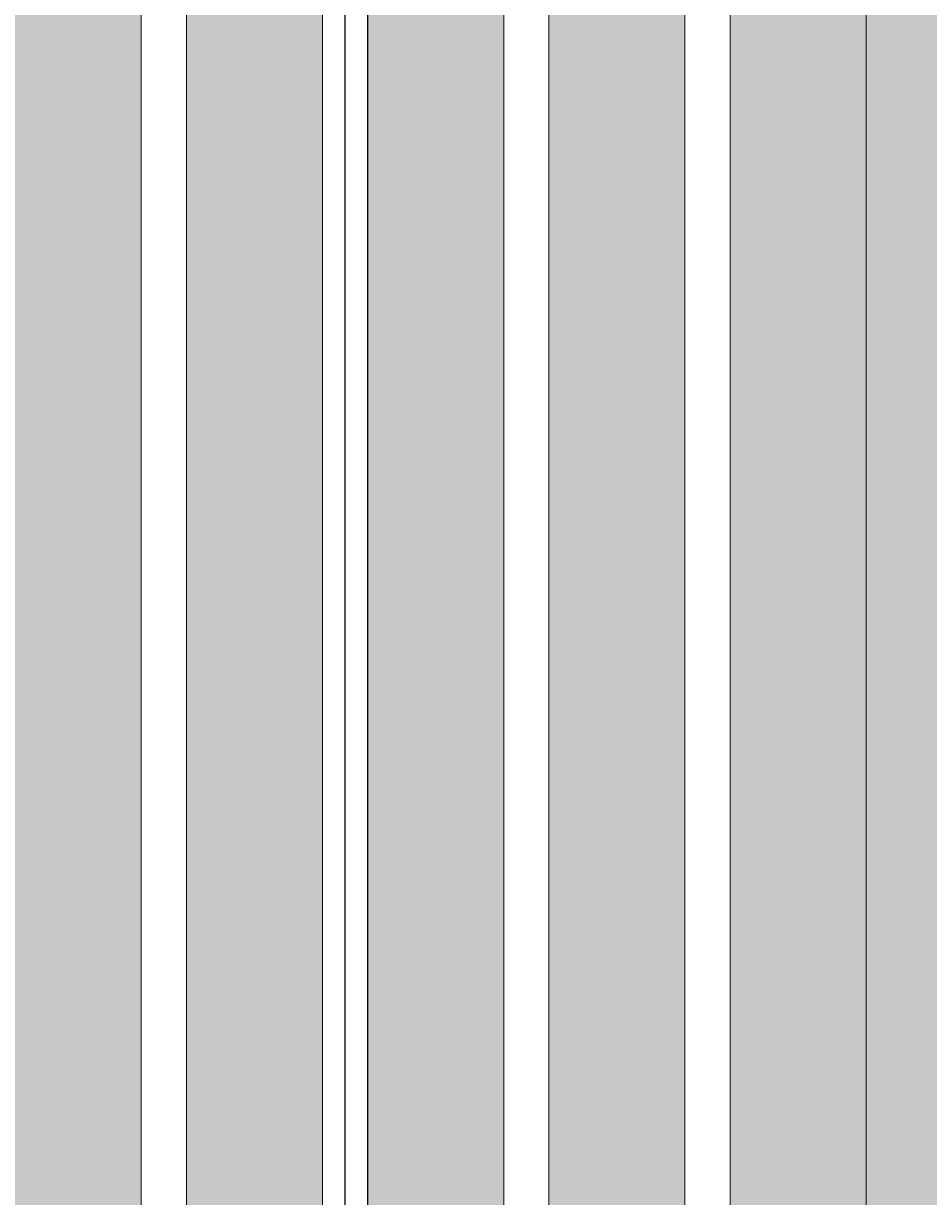
# Model space of a CAD drawing. Units: inches. Extents: x 4508 to 4723, y 847 to 1020.
# Tile 12 of 32: x 4570 to 4590, y 931 to 956. Entities that reach past the tile are written whole.
import ezdxf

# ---------------------------------------------------------------- set-up
doc = ezdxf.new("R2010")
doc.units = ezdxf.units.IN
for name, color, linetype, lineweight in [('A-ANNO-DIMS', 2, 'Continuous', 18), ('A-WALL-FINS', 30, 'Continuous', 18), ('A-WALL-PATT', 254, 'Continuous', 13)]:
    doc.layers.add(name, color=color, linetype=linetype, lineweight=lineweight)
doc.styles.get("Standard").update_dxf_attribs({"font": 'arial.ttf'})
doc.dimstyles.get("Standard").update_dxf_attribs({"dimtxt": 0.18, "dimasz": 0.18, "dimexe": 0.18, "dimexo": 0.0625, "dimgap": 0.09, "dimtad": 0, "dimtih": 1, "dimtoh": 1, "dimdec": 4, "dimzin": 0, "dimdsep": 46, "dimtxsty": 'Standard', "dimcen": 0.09, "dimadec": 0, "dimazin": 0, "dimtfac": 1, "dimtdec": 4, "dimtofl": 0, "dimtmove": 0, "dimatfit": 3, "dimfxl": 1, "dimtolj": 1, "dimtzin": 0, "dimarcsym": 0})

# ---------------------------------------------------------------- blocks, each defined once
blk = doc.blocks.new('*D27')
at = {"layer": 'A-ANNO-DIMS', "color": 0, "lineweight": -2, "transparency": 16777216}
for p, q in [((4550.994, 903.809), (4550.994, 1002.877)), ((4577.494, 903.809), (4577.494, 1002.877)), ((4551.174, 1002.697), (4563.918, 1002.697)), ((4577.314, 1002.697), (4564.57, 1002.697))]:
    blk.add_line(p, q, dxfattribs=at)
at = {"layer": 'A-ANNO-DIMS', "color": 0, "lineweight": 9, "transparency": 16777216}
for points in [[(4551.174, 1002.727), (4551.174, 1002.667), (4550.994, 1002.697)], [(4577.314, 1002.727), (4577.314, 1002.667), (4577.494, 1002.697)]]:
    blk.add_solid(points, dxfattribs=at)
at = {"layer": 'Defpoints', "color": 0, "lineweight": 9, "transparency": 16777216}
for p in [(4577.494, 1002.697), (4550.994, 903.747), (4577.494, 903.747)]:
    blk.add_point(p, dxfattribs=at)
at = {"layer": 'A-ANNO-DIMS', "color": 0, "transparency": 16777216, "insert": (4564.244, 1002.697), "char_height": 0.18, "attachment_point": 5}
blk.add_mtext('\\A1;26.5', dxfattribs=at)
blk = doc.blocks.new('*D28')
at = {"layer": 'A-ANNO-DIMS', "color": 0, "lineweight": -2, "transparency": 16777216}
for p, q in [((4577.494, 903.809), (4577.494, 1002.877)), ((4577.994, 903.809), (4577.994, 1002.877)), ((4577.314, 1002.697), (4577.134, 1002.697)), ((4578.174, 1002.697), (4578.354, 1002.697))]:
    blk.add_line(p, q, dxfattribs=at)
at = {"layer": 'A-ANNO-DIMS', "color": 0, "lineweight": 9, "transparency": 16777216}
for points in [[(4577.314, 1002.727), (4577.314, 1002.667), (4577.494, 1002.697)], [(4578.174, 1002.727), (4578.174, 1002.667), (4577.994, 1002.697)]]:
    blk.add_solid(points, dxfattribs=at)
at = {"layer": 'Defpoints', "color": 0, "lineweight": 9, "transparency": 16777216}
for p in [(4577.994, 1002.697), (4577.494, 903.747), (4577.994, 903.747)]:
    blk.add_point(p, dxfattribs=at)
at = {"layer": 'A-ANNO-DIMS', "color": 0, "transparency": 16777216, "insert": (4578.608, 1002.697), "char_height": 0.18, "attachment_point": 5}
blk.add_mtext('\\A1;0.5', dxfattribs=at)
blk = doc.blocks.new('*D29')
at = {"layer": 'A-ANNO-DIMS', "color": 0, "lineweight": -2, "transparency": 16777216}
for p, q in [((4577.994, 903.809), (4577.994, 1002.877)), ((4603.994, 903.809), (4603.994, 1002.877)), ((4578.174, 1002.697), (4590.773, 1002.697)), ((4603.814, 1002.697), (4591.214, 1002.697))]:
    blk.add_line(p, q, dxfattribs=at)
at = {"layer": 'A-ANNO-DIMS', "color": 0, "lineweight": 9, "transparency": 16777216}
for points in [[(4578.174, 1002.727), (4578.174, 1002.667), (4577.994, 1002.697)], [(4603.814, 1002.727), (4603.814, 1002.667), (4603.994, 1002.697)]]:
    blk.add_solid(points, dxfattribs=at)
at = {"layer": 'Defpoints', "color": 0, "lineweight": 9, "transparency": 16777216}
for p in [(4603.994, 1002.697), (4577.994, 903.747), (4603.994, 903.747)]:
    blk.add_point(p, dxfattribs=at)
at = {"layer": 'A-ANNO-DIMS', "color": 0, "transparency": 16777216, "insert": (4590.994, 1002.697), "char_height": 0.18, "attachment_point": 5}
blk.add_mtext('\\A1;26', dxfattribs=at)

msp = doc.modelspace()

# ---------------------------------------------------------------- hatches: boundary and pattern name
at = {"layer": 'A-WALL-PATT', "transparency": 33554681}
h = msp.add_hatch(color=256, dxfattribs=at)
h.dxf.hatch_style = 1
h.paths.add_polyline_path([(4552.9938, 994.7469), (4549.9938, 994.7469), (4549.9938, 904.7469), (4552.9938, 904.7469)])
h.paths.add_polyline_path([(4556.9938, 994.7469), (4553.9938, 994.7469), (4553.9938, 904.7469), (4556.9938, 904.7469)])
h.paths.add_polyline_path([(4560.9938, 994.7469), (4557.9938, 994.7469), (4557.9938, 904.7469), (4560.9938, 904.7469)])
h.paths.add_polyline_path([(4564.9938, 994.7469), (4561.9938, 994.7469), (4561.9938, 904.7469), (4564.9938, 904.7469)])
h.paths.add_polyline_path([(4568.9938, 994.7469), (4565.9938, 994.7469), (4565.9938, 904.7469), (4568.9938, 904.7469)])
h.paths.add_polyline_path([(4572.9938, 994.7469), (4569.9938, 994.7469), (4569.9938, 904.7469), (4572.9938, 904.7469)])
h.paths.add_polyline_path([(4576.9938, 994.7469), (4573.9938, 994.7469), (4573.9938, 904.7469), (4576.9938, 904.7469)])
h.paths.add_polyline_path([(4580.9938, 994.7469), (4577.9938, 994.7469), (4577.9938, 904.7469), (4580.9938, 904.7469)])
h.paths.add_polyline_path([(4584.9938, 994.7469), (4581.9938, 994.7469), (4581.9938, 904.7469), (4584.9938, 904.7469)])
at = {"layer": 'A-WALL-PATT', "transparency": 33554508}
h = msp.add_hatch(color=256, dxfattribs=at)
h.dxf.hatch_style = 1
h.paths.add_polyline_path([(4661.6706, 954.043, -0.3739004), (4658.5765, 957.6021, -1), (4665.7646, 957.6021, -0.3739004), (4662.6706, 954.043), (4662.6706, 944.4021, -0.2114781), (4670.3062, 945.0869), (4670.3062, 968.0592, -0.4632086), (4663.3246, 973.9783, -0.4632086), (4670.3062, 979.8975), (4670.3062, 994.7469), (4588.9938, 994.7469), (4588.9938, 904.7469), (4657.9938, 904.7469), (4657.9938, 886.7469), (4549.9938, 886.7469), (4549.9938, 878.7469), (4693.9938, 878.7469), (4693.9938, 994.7469), (4671.8062, 994.7469), (4671.8062, 979.4411, -0.2941682), (4675.3246, 973.9783, -0.2941682), (4671.8062, 968.5156), (4671.8062, 944.4278, -0.2741114), (4676.7298, 936.1217, -0.2741114), (4671.8062, 927.8155), (4671.8062, 907.6998, -0.3779645), (4677.0562, 901.7469, -0.3779645), (4671.8062, 895.7939), (4671.8062, 883.7469), (4670.3062, 883.7469), (4670.3062, 895.7939, -0.3779645), (4665.0562, 901.7469, -0.3779645), (4670.3062, 907.6998), (4670.3062, 927.1564, -0.2114781), (4662.6706, 927.8412), (4662.6706, 918.2003, -0.3739004), (4665.7646, 914.6412, -1), (4658.5765, 914.6412, -0.3739004), (4661.6706, 918.2003), (4661.6706, 928.4807, -0.2391825), (4657.7936, 936.1217, -0.2391825), (4661.6706, 943.7626)])
at = {"layer": 'A-WALL-PATT', "transparency": 33554681}
h = msp.add_hatch(color=256, dxfattribs=at)
h.dxf.hatch_style = 1
h.paths.add_polyline_path([(4588.9938, 994.7469), (4585.9938, 994.7469), (4585.9938, 904.7469), (4588.9938, 904.7469)])

# ---------------------------------------------------------------- linework, layer by layer
at = {"layer": 'A-WALL-FINS'}
for p, q in [((4572.9938, 904.7469), (4572.9938, 994.7469)), ((4573.9938, 904.7469), (4573.9938, 994.7469)), ((4576.9938, 904.7469), (4576.9938, 994.7469)), ((4577.9938, 904.7469), (4577.9938, 994.7469)), ((4580.9938, 904.7469), (4580.9938, 994.7469)), ((4581.9938, 904.7469), (4581.9938, 994.7469)), ((4584.9938, 904.7469), (4584.9938, 994.7469)), ((4585.9938, 904.7469), (4585.9938, 994.7469)), ((4588.9938, 904.7469), (4588.9938, 994.7469))]:
    msp.add_line(p, q, dxfattribs=at)

# ---------------------------------------------------------------- dimensions: what is measured, and where the dimension line sits
at = {"layer": 'A-ANNO-DIMS'}
for base, p1, p2, override, picture, middle in [((4577.4938, 1002.6969), (4550.9938, 903.7469), (4577.4938, 903.7469), {"dimdec": 1, "dimlfac": 1, "dimrnd": 0, "dimzin": 0, "dimdsep": 46, "dimlunit": 2}, '*D27', (4564.2438, 1002.6969)), ((4577.9938, 1002.6969), (4577.4938, 903.7469), (4577.9938, 903.7469), {"dimdec": 1, "dimlfac": 1, "dimrnd": 0, "dimzin": 0, "dimdsep": 46, "dimlunit": 2}, '*D28', (4578.6083, 1002.6969)), ((4603.9938, 1002.6969), (4577.9938, 903.7469), (4603.9938, 903.7469), {"dimdec": 0, "dimlfac": 1, "dimrnd": 0, "dimzin": 0, "dimdsep": 46, "dimlunit": 2}, '*D29', (4590.9938, 1002.6969))]:
    dim = msp.add_linear_dim(base=base, p1=p1, p2=p2, dimstyle='Standard', override=override, dxfattribs=at)
    dim.commit()
    dim.dimension.update_dxf_attribs({"geometry": picture, "text_midpoint": middle})

doc.saveas('drawing.dxf')
